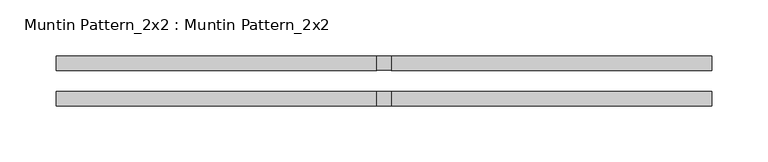
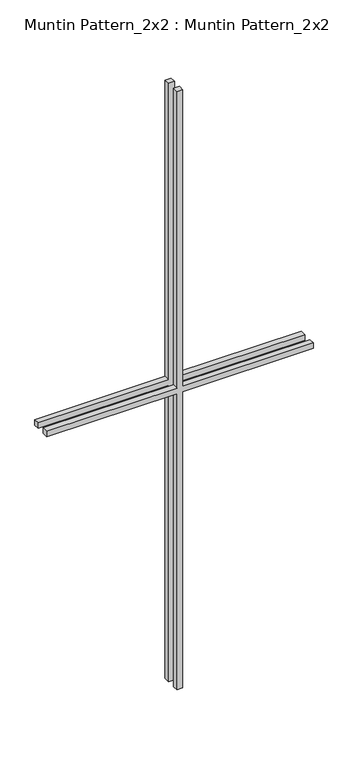
"""IFC4 building model written with IfcOpenShell, lengths in millimetres: proxy geometry, Muntin Pattern_2x2 : Muntin Pattern_2x2."""

from ifc_helpers import new_model, si_unit, frame, origin, place, context, project, spatial, polyline, outline, extrude, source, transform, mapped, element, save


def muntin_pattern_2x2_muntin_pattern_2x2_a6c43cb1(model_context):
    return source(origin(), model_context, "Body", "SweptSolid", [
        extrude(outline(polyline([(698.5, -6.35), (698.5, -292.1), (685.8, -292.1), (685.8, -6.35), (0.0, -6.35), (0.0, 6.35), (685.8, 6.35), (685.8, 292.1), (698.5, 292.1), (698.5, 6.35), (1384.3, 6.35), (1384.3, -6.35), (698.5, -6.35)])), frame((0.0, -22.225, 0.0), z_axis=(0.0, 1.0, 0.0), x_axis=(0.0, 0.0, 1.0)), (0.0, 0.0, 1.0), 12.7),
        extrude(outline(polyline([(698.5, -6.35), (698.5, -292.1), (685.8, -292.1), (685.8, -6.35), (0.0, -6.35), (0.0, 6.35), (685.8, 6.35), (685.8, 292.1), (698.5, 292.1), (698.5, 6.35), (1384.3, 6.35), (1384.3, -6.35), (698.5, -6.35)])), frame((0.0, 9.525, 0.0), z_axis=(0.0, 1.0, 0.0), x_axis=(0.0, 0.0, 1.0)), (0.0, 0.0, 1.0), 12.7),
    ])


if __name__ == "__main__":
    model = new_model("IFC4")
    model_context = context("Model", 3, world=origin())
    ifc_project = project(units=[si_unit("LENGTHUNIT", "METRE", prefix="MILLI")], contexts=[model_context])
    site = spatial("IfcSite", under=ifc_project)
    building = spatial("IfcBuilding", under=site)
    placement = place(None, origin())
    muntin_pattern_2x2_muntin_pattern_2x2_shape = muntin_pattern_2x2_muntin_pattern_2x2_a6c43cb1(model_context)
    element("IfcBuildingElementProxy", 1, Name="Muntin Pattern_2x2 : Muntin Pattern_2x2", ObjectType="Muntin Pattern_2x2 : Muntin Pattern_2x2", at=placement, inside=building, context=model_context, shape_type="MappedRepresentation", body=[
        mapped(muntin_pattern_2x2_muntin_pattern_2x2_shape, transform((0.0, 0.0, 0.0), x_axis=(1.0, 0.0, 0.0), y_axis=(0.0, 1.0, 0.0), z_axis=(0.0, 0.0, 1.0))),
    ])
    save(model, "model.ifc")

# Revit data of these elements
# Type "Muntin Pattern_2x2 : Muntin Pattern_2x2"
#   Width [instance default] = 4' - 0"
#   Thickness = 0' - 0 1/2"
#   Height [instance default] = 4' - 0"
#   Distance = 0' - 0 3/4"
#   Interior Material [instance default] = none
#   Exterior Material [instance default] = none
#   Default Elevation = 0
# Element 1 (IfcBuildingElementProxy, "Muntin Pattern_2x2 : Muntin Pattern_2x2")
#   Width = 1' - 11"
#   Height = 4' - 6 1/2"
#   Interior Material = Wood - Stained
#   Exterior Material = Clad - White
#   Materials on its faces: "Clad - White", "Wood - Stained"
# Materials
#   "Clad - White": class "Wood", colour RGB 242 242 238, transparency 0, Cost = 0
#   "Wood - Stained": class "Wood", colour RGB 224 178 126, transparency 0, Cost = 0
